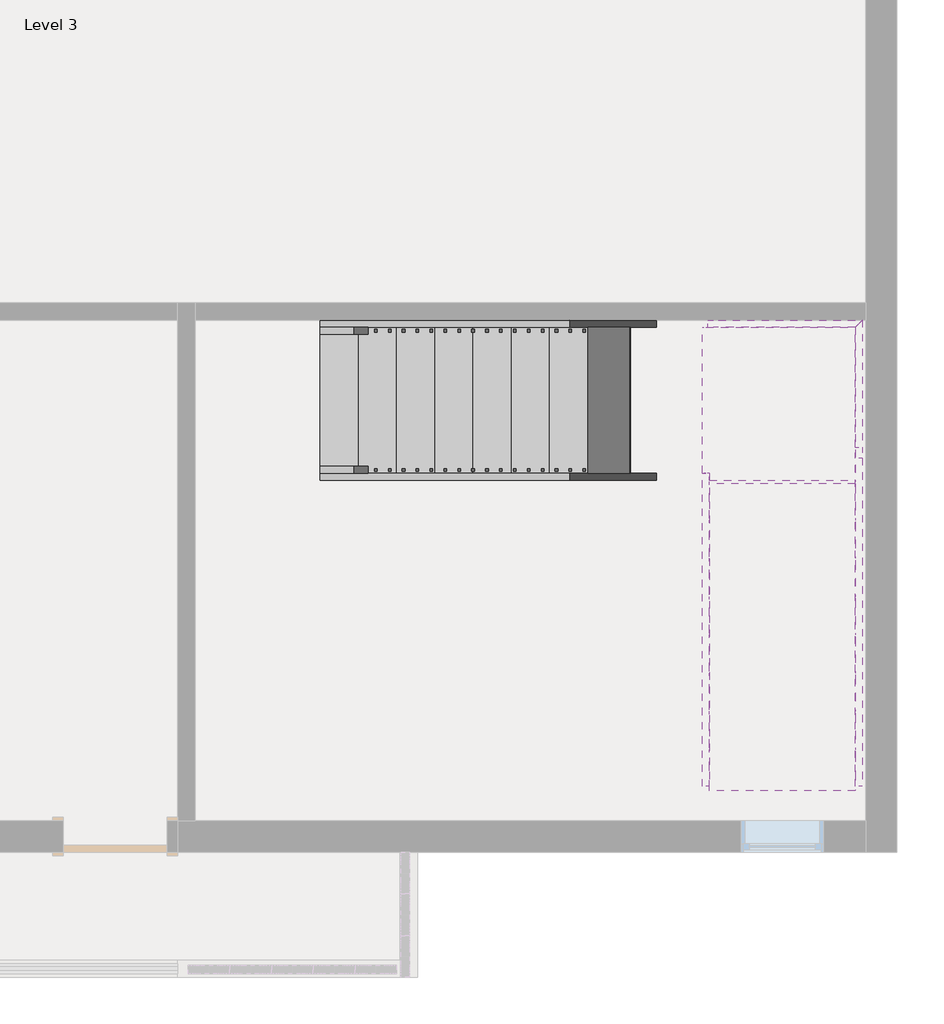
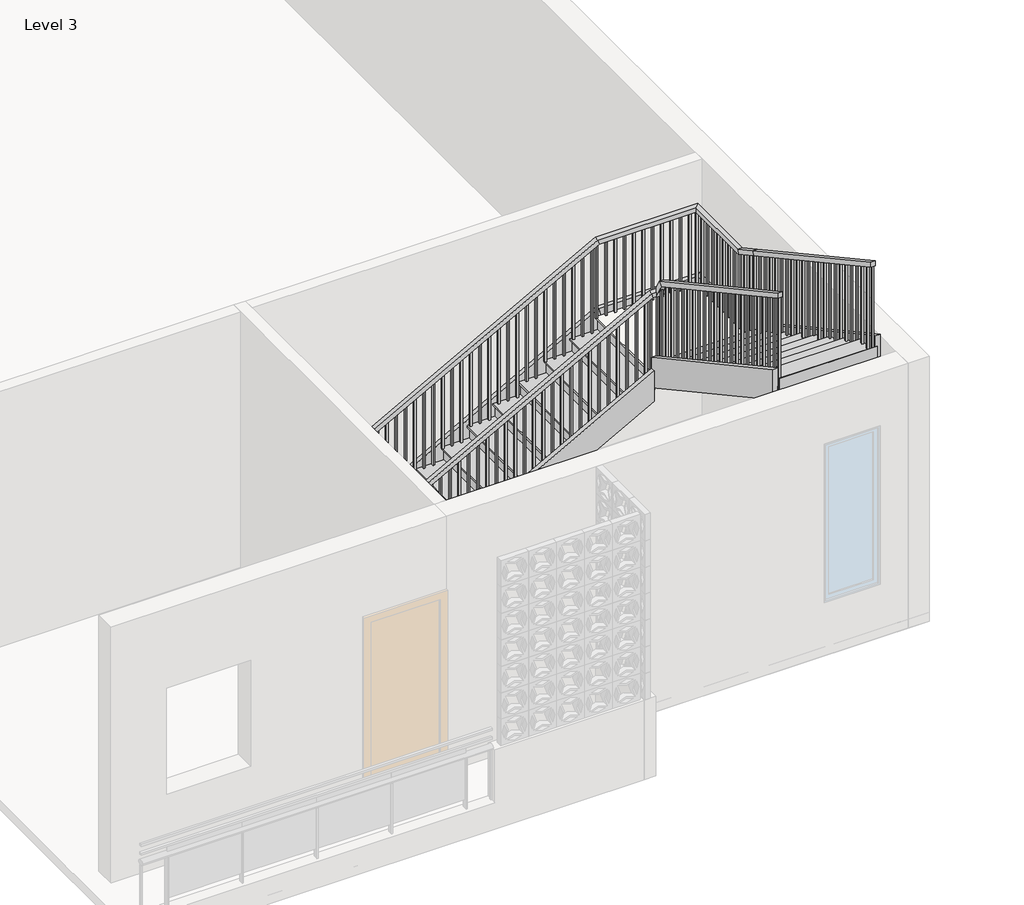
# One storey, part 2 of 2: 6 members, 2 railings, 2 stair flights, 1 slab.
"""IFC4 building model written with IfcOpenShell, lengths in millimetres."""

from ifc_helpers import new_model, si_unit, frame, origin, place, context, project, spatial, polyline, outline, extrude, faceted_brep, transform, mapped, element, save
from components import non_monolithic_landing_ee32a08e, stair_flight_b15b2b3c, stair_flight_a6ac55d9

model = new_model("IFC4")

# Units and contexts
model_context = context("Model", 3, world=origin())
ifc_project = project(units=[si_unit("LENGTHUNIT", "METRE", prefix="MILLI")], contexts=[model_context])

# Site, building, storey
site = spatial("IfcSite", under=ifc_project)
building = spatial("IfcBuilding", under=site)
storey = spatial("IfcBuildingStorey", under=building, Name="Level 3", Elevation=6096.0)

# Members
placement = place(None, origin())
element("IfcMember", 1, ObjectType="Stringer - 2\" Width", at=placement, inside=storey, context=model_context, shape_type="SweptSolid", body=[
    extrude(outline(polyline([(6302.7436667, -459.26646), (6096.0, -459.26646), (6096.0, -201.7743401), (7543.8, 2452.5256599), (7848.6, 2374.8034844), (6302.7436667, -459.26646)])), frame((0.0, -782.3834702, 0.0), z_axis=(0.0, 1.0, 0.0), x_axis=(0.0, 0.0, 1.0)), (0.0, 0.0, 1.0), 50.8),
])
element("IfcMember", 2, ObjectType="Stringer - 2\" Width", at=placement, inside=storey, context=model_context, shape_type="SweptSolid", body=[
    extrude(outline(polyline([(6302.7436667, -459.26646), (6096.0, -459.26646), (6096.0, -201.7743401), (7479.5497528, 2334.73354), (7826.7436667, 2334.73354), (6302.7436667, -459.26646)])), frame((0.0, -1899.9834702, 0.0), z_axis=(0.0, 1.0, 0.0), x_axis=(0.0, 0.0, 1.0)), (0.0, 0.0, 1.0), 50.8),
])
element("IfcMember", 3, ObjectType="Stringer - 2\" Width", at=placement, inside=storey, context=model_context, shape_type="SweptSolid", body=[
    extrude(outline(polyline([(-1660.6534146, 7848.6), (-1738.3755901, 7543.8), (-4135.1834702, 8851.1497528), (-4135.1834702, 9198.3436667), (-1660.6534146, 7848.6)])), frame((3452.33354, 0.0, 0.0), z_axis=(1.0, 0.0, 0.0), x_axis=(0.0, 1.0, 0.0)), (0.0, 0.0, 1.0), 50.8),
])
element("IfcMember", 4, ObjectType="Stringer - 2\" Width", at=placement, inside=storey, context=model_context, shape_type="SweptSolid", body=[
    extrude(outline(polyline([(-1849.1834702, 7951.4345758), (-1849.1834702, 7604.2406619), (-4135.1834702, 8851.1497528), (-4135.1834702, 9198.3436667), (-1849.1834702, 7951.4345758)])), frame((2334.73354, 0.0, 0.0), z_axis=(1.0, 0.0, 0.0), x_axis=(0.0, 1.0, 0.0)), (0.0, 0.0, 1.0), 50.8),
])
element("IfcMember", 5, ObjectType="Stringer - 2\" Width", at=placement, inside=storey, context=model_context, shape_type="Brep", body=[
    faceted_brep([(3452.33354, -1660.6534146, 7848.6), (3503.13354, -1660.6534146, 7848.6), (3503.13354, -731.5834702, 7848.6), (3452.33354, -782.3834702, 7848.6), (3452.33354, -1738.3755901, 7543.8), (3452.33354, -782.3834702, 7543.8), (3503.13354, -1738.3755901, 7543.8), (3503.13354, -731.5834702, 7543.8)], [[[0, 1, 2, 3]], [[4, 0, 3, 5]], [[6, 4, 5, 7]], [[1, 6, 7, 2]], [[1, 0, 4, 6]], [[2, 7, 5, 3]]]),
])
element("IfcMember", 6, ObjectType="Stringer - 2\" Width", at=placement, inside=storey, context=model_context, shape_type="Brep", body=[
    faceted_brep([(3452.33354, -782.3834702, 7848.6), (3503.13354, -731.5834702, 7848.6), (2374.8034844, -731.5834702, 7848.6), (2374.8034844, -782.3834702, 7848.6), (3452.33354, -782.3834702, 7543.8), (2452.5256599, -782.3834702, 7543.8), (3503.13354, -731.5834702, 7543.8), (2452.5256599, -731.5834702, 7543.8)], [[[0, 1, 2, 3]], [[4, 0, 3, 5]], [[6, 4, 5, 7]], [[1, 6, 7, 2]], [[1, 0, 4, 6]], [[2, 7, 5, 3]]]),
])

# Railings
element("IfcRailing", 7, ObjectType="Handrail - Rectangular", at=placement, inside=storey, context=model_context, shape_type="SolidModel", body=[
    faceted_brep([(-459.26646, -1798.3834702, 7162.8), (-459.26646, -1798.3834702, 7104.9343477), (-459.26646, -1849.1834702, 7104.9343477), (-459.26646, -1849.1834702, 7162.8), (2334.73354, -1798.3834702, 8686.8), (2347.687236, -1798.3834702, 8636.0), (2347.687236, -1849.1834702, 8636.0), (2334.73354, -1849.1834702, 8686.8), (2436.33354, -1798.3834702, 8686.8), (2436.33354, -1849.1834702, 8686.8), (2436.33354, -1849.1834702, 8636.0), (2436.33354, -1798.3834702, 8636.0)], [[[0, 1, 2, 3]], [[1, 0, 4, 5]], [[2, 1, 5, 6]], [[3, 2, 6, 7]], [[0, 3, 7, 4]], [[8, 9, 10, 11]], [[5, 4, 8, 11]], [[6, 5, 11, 10]], [[7, 6, 10, 9]], [[4, 7, 9, 8]]]),
    faceted_brep([(2436.33354, -1849.1834702, 8737.6), (2436.33354, -1849.1834702, 8624.0077467), (2385.53354, -1849.1834702, 8624.0077467), (2385.53354, -1849.1834702, 8737.6), (2436.33354, -1899.9834702, 8839.2), (2436.33354, -1938.2955084, 8802.231823), (2385.53354, -1938.2955084, 8802.231823), (2385.53354, -1899.9834702, 8839.2), (2436.33354, -4135.1834702, 10058.4), (2385.53354, -4135.1834702, 10058.4), (2385.53354, -4135.1834702, 10000.5343477), (2436.33354, -4135.1834702, 10000.5343477)], [[[0, 1, 2, 3]], [[1, 0, 4, 5]], [[2, 1, 5, 6]], [[3, 2, 6, 7]], [[0, 3, 7, 4]], [[8, 9, 10, 11]], [[5, 4, 8, 11]], [[6, 5, 11, 10]], [[7, 6, 10, 9]], [[4, 7, 9, 8]]]),
    extrude(outline(polyline([(-4043.1084702, 9950.3116204), (-4024.0584702, 9939.9207113), (-4024.0584702, 8991.6), (-4043.1084702, 8991.6), (-4043.1084702, 9950.3116204)])), frame((2401.40854, 0.0, 0.0), z_axis=(1.0, 0.0, 0.0), x_axis=(0.0, 1.0, 0.0)), (0.0, 0.0, 1.0), 19.05),
    extrude(outline(polyline([(-3941.5084702, 9894.8934386), (-3922.4584702, 9884.5025295), (-3922.4584702, 8991.6), (-3941.5084702, 8991.6), (-3941.5084702, 9894.8934386)])), frame((2401.40854, 0.0, 0.0), z_axis=(1.0, 0.0, 0.0), x_axis=(0.0, 1.0, 0.0)), (0.0, 0.0, 1.0), 19.05),
    extrude(outline(polyline([(-3839.9084702, 9839.4752568), (-3820.8584702, 9829.0843477), (-3820.8584702, 8839.2), (-3839.9084702, 8839.2), (-3839.9084702, 9839.4752568)])), frame((2401.40854, 0.0, 0.0), z_axis=(1.0, 0.0, 0.0), x_axis=(0.0, 1.0, 0.0)), (0.0, 0.0, 1.0), 19.05),
    extrude(outline(polyline([(-3738.3084702, 9784.0570749), (-3719.2584702, 9773.6661659), (-3719.2584702, 8839.2), (-3738.3084702, 8839.2), (-3738.3084702, 9784.0570749)])), frame((2401.40854, 0.0, 0.0), z_axis=(1.0, 0.0, 0.0), x_axis=(0.0, 1.0, 0.0)), (0.0, 0.0, 1.0), 19.05),
    extrude(outline(polyline([(-3636.7084702, 9728.6388931), (-3617.6584702, 9718.247984), (-3617.6584702, 8839.2), (-3636.7084702, 8839.2), (-3636.7084702, 9728.6388931)])), frame((2401.40854, 0.0, 0.0), z_axis=(1.0, 0.0, 0.0), x_axis=(0.0, 1.0, 0.0)), (0.0, 0.0, 1.0), 19.05),
    extrude(outline(polyline([(-3535.1084702, 9673.2207113), (-3516.0584702, 9662.8298022), (-3516.0584702, 8686.8), (-3535.1084702, 8686.8), (-3535.1084702, 9673.2207113)])), frame((2401.40854, 0.0, 0.0), z_axis=(1.0, 0.0, 0.0), x_axis=(0.0, 1.0, 0.0)), (0.0, 0.0, 1.0), 19.05),
    extrude(outline(polyline([(-3433.5084702, 9617.8025295), (-3414.4584702, 9607.4116204), (-3414.4584702, 8686.8), (-3433.5084702, 8686.8), (-3433.5084702, 9617.8025295)])), frame((2401.40854, 0.0, 0.0), z_axis=(1.0, 0.0, 0.0), x_axis=(0.0, 1.0, 0.0)), (0.0, 0.0, 1.0), 19.05),
    extrude(outline(polyline([(-3331.9084702, 9562.3843477), (-3312.8584702, 9551.9934386), (-3312.8584702, 8686.8), (-3331.9084702, 8686.8), (-3331.9084702, 9562.3843477)])), frame((2401.40854, 0.0, 0.0), z_axis=(1.0, 0.0, 0.0), x_axis=(0.0, 1.0, 0.0)), (0.0, 0.0, 1.0), 19.05),
    extrude(outline(polyline([(-3230.3084702, 9506.9661659), (-3211.2584702, 9496.5752568), (-3211.2584702, 8534.4), (-3230.3084702, 8534.4), (-3230.3084702, 9506.9661659)])), frame((2401.40854, 0.0, 0.0), z_axis=(1.0, 0.0, 0.0), x_axis=(0.0, 1.0, 0.0)), (0.0, 0.0, 1.0), 19.05),
    extrude(outline(polyline([(-3128.7084702, 9451.547984), (-3109.6584702, 9441.1570749), (-3109.6584702, 8534.4), (-3128.7084702, 8534.4), (-3128.7084702, 9451.547984)])), frame((2401.40854, 0.0, 0.0), z_axis=(1.0, 0.0, 0.0), x_axis=(0.0, 1.0, 0.0)), (0.0, 0.0, 1.0), 19.05),
    extrude(outline(polyline([(-3027.1084702, 9396.1298022), (-3008.0584702, 9385.7388931), (-3008.0584702, 8534.4), (-3027.1084702, 8534.4), (-3027.1084702, 9396.1298022)])), frame((2401.40854, 0.0, 0.0), z_axis=(1.0, 0.0, 0.0), x_axis=(0.0, 1.0, 0.0)), (0.0, 0.0, 1.0), 19.05),
    extrude(outline(polyline([(-2925.5084702, 9340.7116204), (-2906.4584702, 9330.3207113), (-2906.4584702, 8382.0), (-2925.5084702, 8382.0), (-2925.5084702, 9340.7116204)])), frame((2401.40854, 0.0, 0.0), z_axis=(1.0, 0.0, 0.0), x_axis=(0.0, 1.0, 0.0)), (0.0, 0.0, 1.0), 19.05),
    extrude(outline(polyline([(-2823.9084702, 9285.2934386), (-2804.8584702, 9274.9025295), (-2804.8584702, 8382.0), (-2823.9084702, 8382.0), (-2823.9084702, 9285.2934386)])), frame((2401.40854, 0.0, 0.0), z_axis=(1.0, 0.0, 0.0), x_axis=(0.0, 1.0, 0.0)), (0.0, 0.0, 1.0), 19.05),
    extrude(outline(polyline([(-2722.3084702, 9229.8752568), (-2703.2584702, 9219.4843477), (-2703.2584702, 8229.6), (-2722.3084702, 8229.6), (-2722.3084702, 9229.8752568)])), frame((2401.40854, 0.0, 0.0), z_axis=(1.0, 0.0, 0.0), x_axis=(0.0, 1.0, 0.0)), (0.0, 0.0, 1.0), 19.05),
    extrude(outline(polyline([(-2620.7084702, 9174.4570749), (-2601.6584702, 9164.0661659), (-2601.6584702, 8229.6), (-2620.7084702, 8229.6), (-2620.7084702, 9174.4570749)])), frame((2401.40854, 0.0, 0.0), z_axis=(1.0, 0.0, 0.0), x_axis=(0.0, 1.0, 0.0)), (0.0, 0.0, 1.0), 19.05),
    extrude(outline(polyline([(-2519.1084702, 9119.0388931), (-2500.0584702, 9108.647984), (-2500.0584702, 8229.6), (-2519.1084702, 8229.6), (-2519.1084702, 9119.0388931)])), frame((2401.40854, 0.0, 0.0), z_axis=(1.0, 0.0, 0.0), x_axis=(0.0, 1.0, 0.0)), (0.0, 0.0, 1.0), 19.05),
    extrude(outline(polyline([(-2417.5084702, 9063.6207113), (-2398.4584702, 9053.2298022), (-2398.4584702, 8077.2), (-2417.5084702, 8077.2), (-2417.5084702, 9063.6207113)])), frame((2401.40854, 0.0, 0.0), z_axis=(1.0, 0.0, 0.0), x_axis=(0.0, 1.0, 0.0)), (0.0, 0.0, 1.0), 19.05),
    extrude(outline(polyline([(-2315.9084702, 9008.2025295), (-2296.8584702, 8997.8116204), (-2296.8584702, 8077.2), (-2315.9084702, 8077.2), (-2315.9084702, 9008.2025295)])), frame((2401.40854, 0.0, 0.0), z_axis=(1.0, 0.0, 0.0), x_axis=(0.0, 1.0, 0.0)), (0.0, 0.0, 1.0), 19.05),
    extrude(outline(polyline([(-2214.3084702, 8952.7843477), (-2195.2584702, 8942.3934386), (-2195.2584702, 8077.2), (-2214.3084702, 8077.2), (-2214.3084702, 8952.7843477)])), frame((2401.40854, 0.0, 0.0), z_axis=(1.0, 0.0, 0.0), x_axis=(0.0, 1.0, 0.0)), (0.0, 0.0, 1.0), 19.05),
    extrude(outline(polyline([(-2112.7084702, 8897.3661659), (-2093.6584702, 8886.9752568), (-2093.6584702, 7924.8), (-2112.7084702, 7924.8), (-2112.7084702, 8897.3661659)])), frame((2401.40854, 0.0, 0.0), z_axis=(1.0, 0.0, 0.0), x_axis=(0.0, 1.0, 0.0)), (0.0, 0.0, 1.0), 19.05),
    extrude(outline(polyline([(-2011.1084702, 8841.947984), (-1992.0584702, 8831.5570749), (-1992.0584702, 7924.8), (-2011.1084702, 7924.8), (-2011.1084702, 8841.947984)])), frame((2401.40854, 0.0, 0.0), z_axis=(1.0, 0.0, 0.0), x_axis=(0.0, 1.0, 0.0)), (0.0, 0.0, 1.0), 19.05),
    extrude(outline(polyline([(8606.4207113, 2293.45854), (8596.0298022, 2274.40854), (7620.0, 2274.40854), (7620.0, 2293.45854), (8606.4207113, 2293.45854)])), frame((0.0, -1833.3084702, 0.0), z_axis=(0.0, 1.0, 0.0), x_axis=(0.0, 0.0, 1.0)), (0.0, 0.0, 1.0), 19.05),
    extrude(outline(polyline([(8551.0025295, 2191.85854), (8540.6116204, 2172.80854), (7620.0, 2172.80854), (7620.0, 2191.85854), (8551.0025295, 2191.85854)])), frame((0.0, -1833.3084702, 0.0), z_axis=(0.0, 1.0, 0.0), x_axis=(0.0, 0.0, 1.0)), (0.0, 0.0, 1.0), 19.05),
    extrude(outline(polyline([(8495.5843477, 2090.25854), (8485.1934386, 2071.20854), (7620.0, 2071.20854), (7620.0, 2090.25854), (8495.5843477, 2090.25854)])), frame((0.0, -1833.3084702, 0.0), z_axis=(0.0, 1.0, 0.0), x_axis=(0.0, 0.0, 1.0)), (0.0, 0.0, 1.0), 19.05),
    extrude(outline(polyline([(8440.1661659, 1988.65854), (8429.7752568, 1969.60854), (7467.6, 1969.60854), (7467.6, 1988.65854), (8440.1661659, 1988.65854)])), frame((0.0, -1833.3084702, 0.0), z_axis=(0.0, 1.0, 0.0), x_axis=(0.0, 0.0, 1.0)), (0.0, 0.0, 1.0), 19.05),
    extrude(outline(polyline([(8384.747984, 1887.05854), (8374.3570749, 1868.00854), (7467.6, 1868.00854), (7467.6, 1887.05854), (8384.747984, 1887.05854)])), frame((0.0, -1833.3084702, 0.0), z_axis=(0.0, 1.0, 0.0), x_axis=(0.0, 0.0, 1.0)), (0.0, 0.0, 1.0), 19.05),
    extrude(outline(polyline([(8329.3298022, 1785.45854), (8318.9388931, 1766.40854), (7467.6, 1766.40854), (7467.6, 1785.45854), (8329.3298022, 1785.45854)])), frame((0.0, -1833.3084702, 0.0), z_axis=(0.0, 1.0, 0.0), x_axis=(0.0, 0.0, 1.0)), (0.0, 0.0, 1.0), 19.05),
    extrude(outline(polyline([(8273.9116204, 1683.85854), (8263.5207113, 1664.80854), (7315.2, 1664.80854), (7315.2, 1683.85854), (8273.9116204, 1683.85854)])), frame((0.0, -1833.3084702, 0.0), z_axis=(0.0, 1.0, 0.0), x_axis=(0.0, 0.0, 1.0)), (0.0, 0.0, 1.0), 19.05),
    extrude(outline(polyline([(8218.4934386, 1582.25854), (8208.1025295, 1563.20854), (7315.2, 1563.20854), (7315.2, 1582.25854), (8218.4934386, 1582.25854)])), frame((0.0, -1833.3084702, 0.0), z_axis=(0.0, 1.0, 0.0), x_axis=(0.0, 0.0, 1.0)), (0.0, 0.0, 1.0), 19.05),
    extrude(outline(polyline([(8163.0752568, 1480.65854), (8152.6843477, 1461.60854), (7162.8, 1461.60854), (7162.8, 1480.65854), (8163.0752568, 1480.65854)])), frame((0.0, -1833.3084702, 0.0), z_axis=(0.0, 1.0, 0.0), x_axis=(0.0, 0.0, 1.0)), (0.0, 0.0, 1.0), 19.05),
    extrude(outline(polyline([(8107.6570749, 1379.05854), (8097.2661659, 1360.00854), (7162.8, 1360.00854), (7162.8, 1379.05854), (8107.6570749, 1379.05854)])), frame((0.0, -1833.3084702, 0.0), z_axis=(0.0, 1.0, 0.0), x_axis=(0.0, 0.0, 1.0)), (0.0, 0.0, 1.0), 19.05),
    extrude(outline(polyline([(8052.2388931, 1277.45854), (8041.847984, 1258.40854), (7162.8, 1258.40854), (7162.8, 1277.45854), (8052.2388931, 1277.45854)])), frame((0.0, -1833.3084702, 0.0), z_axis=(0.0, 1.0, 0.0), x_axis=(0.0, 0.0, 1.0)), (0.0, 0.0, 1.0), 19.05),
    extrude(outline(polyline([(7996.8207113, 1175.85854), (7986.4298022, 1156.80854), (7010.4, 1156.80854), (7010.4, 1175.85854), (7996.8207113, 1175.85854)])), frame((0.0, -1833.3084702, 0.0), z_axis=(0.0, 1.0, 0.0), x_axis=(0.0, 0.0, 1.0)), (0.0, 0.0, 1.0), 19.05),
    extrude(outline(polyline([(7941.4025295, 1074.25854), (7931.0116204, 1055.20854), (7010.4, 1055.20854), (7010.4, 1074.25854), (7941.4025295, 1074.25854)])), frame((0.0, -1833.3084702, 0.0), z_axis=(0.0, 1.0, 0.0), x_axis=(0.0, 0.0, 1.0)), (0.0, 0.0, 1.0), 19.05),
    extrude(outline(polyline([(7885.9843477, 972.65854), (7875.5934386, 953.60854), (7010.4, 953.60854), (7010.4, 972.65854), (7885.9843477, 972.65854)])), frame((0.0, -1833.3084702, 0.0), z_axis=(0.0, 1.0, 0.0), x_axis=(0.0, 0.0, 1.0)), (0.0, 0.0, 1.0), 19.05),
    extrude(outline(polyline([(7830.5661659, 871.05854), (7820.1752568, 852.00854), (6858.0, 852.00854), (6858.0, 871.05854), (7830.5661659, 871.05854)])), frame((0.0, -1833.3084702, 0.0), z_axis=(0.0, 1.0, 0.0), x_axis=(0.0, 0.0, 1.0)), (0.0, 0.0, 1.0), 19.05),
    extrude(outline(polyline([(7775.147984, 769.45854), (7764.7570749, 750.40854), (6858.0, 750.40854), (6858.0, 769.45854), (7775.147984, 769.45854)])), frame((0.0, -1833.3084702, 0.0), z_axis=(0.0, 1.0, 0.0), x_axis=(0.0, 0.0, 1.0)), (0.0, 0.0, 1.0), 19.05),
    extrude(outline(polyline([(7719.7298022, 667.85854), (7709.3388931, 648.80854), (6858.0, 648.80854), (6858.0, 667.85854), (7719.7298022, 667.85854)])), frame((0.0, -1833.3084702, 0.0), z_axis=(0.0, 1.0, 0.0), x_axis=(0.0, 0.0, 1.0)), (0.0, 0.0, 1.0), 19.05),
    extrude(outline(polyline([(7664.3116204, 566.25854), (7653.9207113, 547.20854), (6705.6, 547.20854), (6705.6, 566.25854), (7664.3116204, 566.25854)])), frame((0.0, -1833.3084702, 0.0), z_axis=(0.0, 1.0, 0.0), x_axis=(0.0, 0.0, 1.0)), (0.0, 0.0, 1.0), 19.05),
    extrude(outline(polyline([(7608.8934386, 464.65854), (7598.5025295, 445.60854), (6705.6, 445.60854), (6705.6, 464.65854), (7608.8934386, 464.65854)])), frame((0.0, -1833.3084702, 0.0), z_axis=(0.0, 1.0, 0.0), x_axis=(0.0, 0.0, 1.0)), (0.0, 0.0, 1.0), 19.05),
    extrude(outline(polyline([(7553.4752568, 363.05854), (7543.0843477, 344.00854), (6553.2, 344.00854), (6553.2, 363.05854), (7553.4752568, 363.05854)])), frame((0.0, -1833.3084702, 0.0), z_axis=(0.0, 1.0, 0.0), x_axis=(0.0, 0.0, 1.0)), (0.0, 0.0, 1.0), 19.05),
    extrude(outline(polyline([(7498.0570749, 261.45854), (7487.6661659, 242.40854), (6553.2, 242.40854), (6553.2, 261.45854), (7498.0570749, 261.45854)])), frame((0.0, -1833.3084702, 0.0), z_axis=(0.0, 1.0, 0.0), x_axis=(0.0, 0.0, 1.0)), (0.0, 0.0, 1.0), 19.05),
    extrude(outline(polyline([(7442.6388931, 159.85854), (7432.247984, 140.80854), (6553.2, 140.80854), (6553.2, 159.85854), (7442.6388931, 159.85854)])), frame((0.0, -1833.3084702, 0.0), z_axis=(0.0, 1.0, 0.0), x_axis=(0.0, 0.0, 1.0)), (0.0, 0.0, 1.0), 19.05),
    extrude(outline(polyline([(7387.2207113, 58.25854), (7376.8298022, 39.20854), (6400.8, 39.20854), (6400.8, 58.25854), (7387.2207113, 58.25854)])), frame((0.0, -1833.3084702, 0.0), z_axis=(0.0, 1.0, 0.0), x_axis=(0.0, 0.0, 1.0)), (0.0, 0.0, 1.0), 19.05),
    extrude(outline(polyline([(7331.8025295, -43.34146), (7321.4116204, -62.39146), (6400.8, -62.39146), (6400.8, -43.34146), (7331.8025295, -43.34146)])), frame((0.0, -1833.3084702, 0.0), z_axis=(0.0, 1.0, 0.0), x_axis=(0.0, 0.0, 1.0)), (0.0, 0.0, 1.0), 19.05),
    extrude(outline(polyline([(7276.3843477, -144.94146), (7265.9934386, -163.99146), (6400.8, -163.99146), (6400.8, -144.94146), (7276.3843477, -144.94146)])), frame((0.0, -1833.3084702, 0.0), z_axis=(0.0, 1.0, 0.0), x_axis=(0.0, 0.0, 1.0)), (0.0, 0.0, 1.0), 19.05),
    extrude(outline(polyline([(7220.9661659, -246.54146), (7210.5752568, -265.59146), (6248.4, -265.59146), (6248.4, -246.54146), (7220.9661659, -246.54146)])), frame((0.0, -1833.3084702, 0.0), z_axis=(0.0, 1.0, 0.0), x_axis=(0.0, 0.0, 1.0)), (0.0, 0.0, 1.0), 19.05),
    extrude(outline(polyline([(7165.547984, -348.14146), (7155.1570749, -367.19146), (6248.4, -367.19146), (6248.4, -348.14146), (7165.547984, -348.14146)])), frame((0.0, -1833.3084702, 0.0), z_axis=(0.0, 1.0, 0.0), x_axis=(0.0, 0.0, 1.0)), (0.0, 0.0, 1.0), 19.05),
    extrude(outline(polyline([(-1909.5084702, 8744.6577467), (-1890.4584702, 8706.5577467), (-1890.4584702, 7772.4), (-1909.5084702, 7772.4), (-1909.5084702, 8744.6577467)])), frame((2401.40854, 0.0, 0.0), z_axis=(1.0, 0.0, 0.0), x_axis=(0.0, 1.0, 0.0)), (0.0, 0.0, 1.0), 19.05),
    extrude(outline(polyline([(2401.40854, -1833.3084702), (2401.40854, -1814.2584702), (2420.45854, -1814.2584702), (2420.45854, -1833.3084702), (2401.40854, -1833.3084702)])), frame((0.0, 0.0, 7772.4), z_axis=(0.0, 0.0, 1.0), x_axis=(1.0, 0.0, 0.0)), (0.0, 0.0, 1.0), 863.6),
    extrude(outline(polyline([(8634.1298022, 2344.25854), (8623.7388931, 2325.20854), (7772.4, 2325.20854), (7772.4, 2344.25854), (8634.1298022, 2344.25854)])), frame((0.0, -1833.3084702, 0.0), z_axis=(0.0, 1.0, 0.0), x_axis=(0.0, 0.0, 1.0)), (0.0, 0.0, 1.0), 19.05),
    extrude(outline(polyline([(-4135.1834702, 10000.5343477), (-4116.1334702, 9990.1434386), (-4116.1334702, 8991.6), (-4135.1834702, 8991.6), (-4135.1834702, 10000.5343477)])), frame((2401.40854, 0.0, 0.0), z_axis=(1.0, 0.0, 0.0), x_axis=(0.0, 1.0, 0.0)), (0.0, 0.0, 1.0), 19.05),
    extrude(outline(polyline([(7115.3252568, -440.21646), (7104.9343477, -459.26646), (6248.4, -459.26646), (6248.4, -440.21646), (7115.3252568, -440.21646)])), frame((0.0, -1833.3084702, 0.0), z_axis=(0.0, 1.0, 0.0), x_axis=(0.0, 0.0, 1.0)), (0.0, 0.0, 1.0), 19.05),
])
element("IfcRailing", 8, ObjectType="Handrail - Rectangular", at=placement, inside=storey, context=model_context, shape_type="SolidModel", body=[
    faceted_brep([(-459.26646, -782.3834702, 7162.8), (-459.26646, -782.3834702, 7104.9343477), (-459.26646, -833.1834702, 7104.9343477), (-459.26646, -833.1834702, 7162.8), (2334.73354, -782.3834702, 8686.8), (2347.687236, -782.3834702, 8636.0), (2347.687236, -833.1834702, 8636.0), (2334.73354, -833.1834702, 8686.8), (3452.33354, -782.3834702, 8686.8), (3452.33354, -782.3834702, 8636.0), (3401.53354, -833.1834702, 8636.0), (3401.53354, -833.1834702, 8686.8), (3452.33354, -1620.5834702, 8686.8), (3452.33354, -1633.5371661, 8636.0), (3401.53354, -1633.5371661, 8636.0), (3401.53354, -1620.5834702, 8686.8), (3452.33354, -1899.9834702, 8839.2), (3452.33354, -1924.3091585, 8794.6029049), (3401.53354, -1924.3091585, 8794.6029049), (3401.53354, -1899.9834702, 8839.2), (3452.33354, -4135.1834702, 10058.4), (3401.53354, -4135.1834702, 10058.4), (3401.53354, -4135.1834702, 10000.5343477), (3452.33354, -4135.1834702, 10000.5343477)], [[[0, 1, 2, 3]], [[1, 0, 4, 5]], [[2, 1, 5, 6]], [[3, 2, 6, 7]], [[0, 3, 7, 4]], [[5, 4, 8, 9]], [[6, 5, 9, 10]], [[7, 6, 10, 11]], [[4, 7, 11, 8]], [[9, 8, 12, 13]], [[10, 9, 13, 14]], [[11, 10, 14, 15]], [[8, 11, 15, 12]], [[13, 12, 16, 17]], [[14, 13, 17, 18]], [[15, 14, 18, 19]], [[12, 15, 19, 16]], [[20, 21, 22, 23]], [[17, 16, 20, 23]], [[18, 17, 23, 22]], [[19, 18, 22, 21]], [[16, 19, 21, 20]]]),
    extrude(outline(polyline([(-4024.0584702, 9939.9207113), (-4024.0584702, 8991.6), (-4043.1084702, 8991.6), (-4043.1084702, 9950.3116204), (-4024.0584702, 9939.9207113)])), frame((3417.40854, 0.0, 0.0), z_axis=(1.0, 0.0, 0.0), x_axis=(0.0, 1.0, 0.0)), (0.0, 0.0, 1.0), 19.05),
    extrude(outline(polyline([(-3922.4584702, 9884.5025295), (-3922.4584702, 8991.6), (-3941.5084702, 8991.6), (-3941.5084702, 9894.8934386), (-3922.4584702, 9884.5025295)])), frame((3417.40854, 0.0, 0.0), z_axis=(1.0, 0.0, 0.0), x_axis=(0.0, 1.0, 0.0)), (0.0, 0.0, 1.0), 19.05),
    extrude(outline(polyline([(-3820.8584702, 9829.0843477), (-3820.8584702, 8839.2), (-3839.9084702, 8839.2), (-3839.9084702, 9839.4752568), (-3820.8584702, 9829.0843477)])), frame((3417.40854, 0.0, 0.0), z_axis=(1.0, 0.0, 0.0), x_axis=(0.0, 1.0, 0.0)), (0.0, 0.0, 1.0), 19.05),
    extrude(outline(polyline([(-3719.2584702, 9773.6661659), (-3719.2584702, 8839.2), (-3738.3084702, 8839.2), (-3738.3084702, 9784.0570749), (-3719.2584702, 9773.6661659)])), frame((3417.40854, 0.0, 0.0), z_axis=(1.0, 0.0, 0.0), x_axis=(0.0, 1.0, 0.0)), (0.0, 0.0, 1.0), 19.05),
    extrude(outline(polyline([(-3617.6584702, 9718.247984), (-3617.6584702, 8839.2), (-3636.7084702, 8839.2), (-3636.7084702, 9728.6388931), (-3617.6584702, 9718.247984)])), frame((3417.40854, 0.0, 0.0), z_axis=(1.0, 0.0, 0.0), x_axis=(0.0, 1.0, 0.0)), (0.0, 0.0, 1.0), 19.05),
    extrude(outline(polyline([(-3516.0584702, 9662.8298022), (-3516.0584702, 8686.8), (-3535.1084702, 8686.8), (-3535.1084702, 9673.2207113), (-3516.0584702, 9662.8298022)])), frame((3417.40854, 0.0, 0.0), z_axis=(1.0, 0.0, 0.0), x_axis=(0.0, 1.0, 0.0)), (0.0, 0.0, 1.0), 19.05),
    extrude(outline(polyline([(-3414.4584702, 9607.4116204), (-3414.4584702, 8686.8), (-3433.5084702, 8686.8), (-3433.5084702, 9617.8025295), (-3414.4584702, 9607.4116204)])), frame((3417.40854, 0.0, 0.0), z_axis=(1.0, 0.0, 0.0), x_axis=(0.0, 1.0, 0.0)), (0.0, 0.0, 1.0), 19.05),
    extrude(outline(polyline([(-3312.8584702, 9551.9934386), (-3312.8584702, 8686.8), (-3331.9084702, 8686.8), (-3331.9084702, 9562.3843477), (-3312.8584702, 9551.9934386)])), frame((3417.40854, 0.0, 0.0), z_axis=(1.0, 0.0, 0.0), x_axis=(0.0, 1.0, 0.0)), (0.0, 0.0, 1.0), 19.05),
    extrude(outline(polyline([(-3211.2584702, 9496.5752568), (-3211.2584702, 8534.4), (-3230.3084702, 8534.4), (-3230.3084702, 9506.9661659), (-3211.2584702, 9496.5752568)])), frame((3417.40854, 0.0, 0.0), z_axis=(1.0, 0.0, 0.0), x_axis=(0.0, 1.0, 0.0)), (0.0, 0.0, 1.0), 19.05),
    extrude(outline(polyline([(-3109.6584702, 9441.1570749), (-3109.6584702, 8534.4), (-3128.7084702, 8534.4), (-3128.7084702, 9451.547984), (-3109.6584702, 9441.1570749)])), frame((3417.40854, 0.0, 0.0), z_axis=(1.0, 0.0, 0.0), x_axis=(0.0, 1.0, 0.0)), (0.0, 0.0, 1.0), 19.05),
    extrude(outline(polyline([(-3008.0584702, 9385.7388931), (-3008.0584702, 8534.4), (-3027.1084702, 8534.4), (-3027.1084702, 9396.1298022), (-3008.0584702, 9385.7388931)])), frame((3417.40854, 0.0, 0.0), z_axis=(1.0, 0.0, 0.0), x_axis=(0.0, 1.0, 0.0)), (0.0, 0.0, 1.0), 19.05),
    extrude(outline(polyline([(-2906.4584702, 9330.3207113), (-2906.4584702, 8382.0), (-2925.5084702, 8382.0), (-2925.5084702, 9340.7116204), (-2906.4584702, 9330.3207113)])), frame((3417.40854, 0.0, 0.0), z_axis=(1.0, 0.0, 0.0), x_axis=(0.0, 1.0, 0.0)), (0.0, 0.0, 1.0), 19.05),
    extrude(outline(polyline([(-2804.8584702, 9274.9025295), (-2804.8584702, 8382.0), (-2823.9084702, 8382.0), (-2823.9084702, 9285.2934386), (-2804.8584702, 9274.9025295)])), frame((3417.40854, 0.0, 0.0), z_axis=(1.0, 0.0, 0.0), x_axis=(0.0, 1.0, 0.0)), (0.0, 0.0, 1.0), 19.05),
    extrude(outline(polyline([(-2703.2584702, 9219.4843477), (-2703.2584702, 8229.6), (-2722.3084702, 8229.6), (-2722.3084702, 9229.8752568), (-2703.2584702, 9219.4843477)])), frame((3417.40854, 0.0, 0.0), z_axis=(1.0, 0.0, 0.0), x_axis=(0.0, 1.0, 0.0)), (0.0, 0.0, 1.0), 19.05),
    extrude(outline(polyline([(-2601.6584702, 9164.0661659), (-2601.6584702, 8229.6), (-2620.7084702, 8229.6), (-2620.7084702, 9174.4570749), (-2601.6584702, 9164.0661659)])), frame((3417.40854, 0.0, 0.0), z_axis=(1.0, 0.0, 0.0), x_axis=(0.0, 1.0, 0.0)), (0.0, 0.0, 1.0), 19.05),
    extrude(outline(polyline([(-2500.0584702, 9108.647984), (-2500.0584702, 8229.6), (-2519.1084702, 8229.6), (-2519.1084702, 9119.0388931), (-2500.0584702, 9108.647984)])), frame((3417.40854, 0.0, 0.0), z_axis=(1.0, 0.0, 0.0), x_axis=(0.0, 1.0, 0.0)), (0.0, 0.0, 1.0), 19.05),
    extrude(outline(polyline([(-2398.4584702, 9053.2298022), (-2398.4584702, 8077.2), (-2417.5084702, 8077.2), (-2417.5084702, 9063.6207113), (-2398.4584702, 9053.2298022)])), frame((3417.40854, 0.0, 0.0), z_axis=(1.0, 0.0, 0.0), x_axis=(0.0, 1.0, 0.0)), (0.0, 0.0, 1.0), 19.05),
    extrude(outline(polyline([(-2296.8584702, 8997.8116204), (-2296.8584702, 8077.2), (-2315.9084702, 8077.2), (-2315.9084702, 9008.2025295), (-2296.8584702, 8997.8116204)])), frame((3417.40854, 0.0, 0.0), z_axis=(1.0, 0.0, 0.0), x_axis=(0.0, 1.0, 0.0)), (0.0, 0.0, 1.0), 19.05),
    extrude(outline(polyline([(-2195.2584702, 8942.3934386), (-2195.2584702, 8077.2), (-2214.3084702, 8077.2), (-2214.3084702, 8952.7843477), (-2195.2584702, 8942.3934386)])), frame((3417.40854, 0.0, 0.0), z_axis=(1.0, 0.0, 0.0), x_axis=(0.0, 1.0, 0.0)), (0.0, 0.0, 1.0), 19.05),
    extrude(outline(polyline([(-2093.6584702, 8886.9752568), (-2093.6584702, 7924.8), (-2112.7084702, 7924.8), (-2112.7084702, 8897.3661659), (-2093.6584702, 8886.9752568)])), frame((3417.40854, 0.0, 0.0), z_axis=(1.0, 0.0, 0.0), x_axis=(0.0, 1.0, 0.0)), (0.0, 0.0, 1.0), 19.05),
    extrude(outline(polyline([(-1992.0584702, 8831.5570749), (-1992.0584702, 7924.8), (-2011.1084702, 7924.8), (-2011.1084702, 8841.947984), (-1992.0584702, 8831.5570749)])), frame((3417.40854, 0.0, 0.0), z_axis=(1.0, 0.0, 0.0), x_axis=(0.0, 1.0, 0.0)), (0.0, 0.0, 1.0), 19.05),
    extrude(outline(polyline([(-1814.2584702, 8734.5752568), (-1814.2584702, 7772.4), (-1833.3084702, 7772.4), (-1833.3084702, 8744.9661659), (-1814.2584702, 8734.5752568)])), frame((3417.40854, 0.0, 0.0), z_axis=(1.0, 0.0, 0.0), x_axis=(0.0, 1.0, 0.0)), (0.0, 0.0, 1.0), 19.05),
    extrude(outline(polyline([(-1712.6584702, 8679.1570749), (-1712.6584702, 7772.4), (-1731.7084702, 7772.4), (-1731.7084702, 8689.547984), (-1712.6584702, 8679.1570749)])), frame((3417.40854, 0.0, 0.0), z_axis=(1.0, 0.0, 0.0), x_axis=(0.0, 1.0, 0.0)), (0.0, 0.0, 1.0), 19.05),
    extrude(outline(polyline([(3436.45854, -1611.0584702), (3436.45854, -1630.1084702), (3417.40854, -1630.1084702), (3417.40854, -1611.0584702), (3436.45854, -1611.0584702)])), frame((0.0, 0.0, 7772.4), z_axis=(0.0, 0.0, 1.0), x_axis=(1.0, 0.0, 0.0)), (0.0, 0.0, 1.0), 863.6),
    extrude(outline(polyline([(3436.45854, -1509.4584702), (3436.45854, -1528.5084702), (3417.40854, -1528.5084702), (3417.40854, -1509.4584702), (3436.45854, -1509.4584702)])), frame((0.0, 0.0, 7772.4), z_axis=(0.0, 0.0, 1.0), x_axis=(1.0, 0.0, 0.0)), (0.0, 0.0, 1.0), 863.6),
    extrude(outline(polyline([(3436.45854, -1407.8584702), (3436.45854, -1426.9084702), (3417.40854, -1426.9084702), (3417.40854, -1407.8584702), (3436.45854, -1407.8584702)])), frame((0.0, 0.0, 7772.4), z_axis=(0.0, 0.0, 1.0), x_axis=(1.0, 0.0, 0.0)), (0.0, 0.0, 1.0), 863.6),
    extrude(outline(polyline([(3436.45854, -1306.2584702), (3436.45854, -1325.3084702), (3417.40854, -1325.3084702), (3417.40854, -1306.2584702), (3436.45854, -1306.2584702)])), frame((0.0, 0.0, 7772.4), z_axis=(0.0, 0.0, 1.0), x_axis=(1.0, 0.0, 0.0)), (0.0, 0.0, 1.0), 863.6),
    extrude(outline(polyline([(3436.45854, -1204.6584702), (3436.45854, -1223.7084702), (3417.40854, -1223.7084702), (3417.40854, -1204.6584702), (3436.45854, -1204.6584702)])), frame((0.0, 0.0, 7772.4), z_axis=(0.0, 0.0, 1.0), x_axis=(1.0, 0.0, 0.0)), (0.0, 0.0, 1.0), 863.6),
    extrude(outline(polyline([(3436.45854, -1103.0584702), (3436.45854, -1122.1084702), (3417.40854, -1122.1084702), (3417.40854, -1103.0584702), (3436.45854, -1103.0584702)])), frame((0.0, 0.0, 7772.4), z_axis=(0.0, 0.0, 1.0), x_axis=(1.0, 0.0, 0.0)), (0.0, 0.0, 1.0), 863.6),
    extrude(outline(polyline([(3436.45854, -1001.4584702), (3436.45854, -1020.5084702), (3417.40854, -1020.5084702), (3417.40854, -1001.4584702), (3436.45854, -1001.4584702)])), frame((0.0, 0.0, 7772.4), z_axis=(0.0, 0.0, 1.0), x_axis=(1.0, 0.0, 0.0)), (0.0, 0.0, 1.0), 863.6),
    extrude(outline(polyline([(3436.45854, -899.8584702), (3436.45854, -918.9084702), (3417.40854, -918.9084702), (3417.40854, -899.8584702), (3436.45854, -899.8584702)])), frame((0.0, 0.0, 7772.4), z_axis=(0.0, 0.0, 1.0), x_axis=(1.0, 0.0, 0.0)), (0.0, 0.0, 1.0), 863.6),
    extrude(outline(polyline([(3341.20854, -798.2584702), (3360.25854, -798.2584702), (3360.25854, -817.3084702), (3341.20854, -817.3084702), (3341.20854, -798.2584702)])), frame((0.0, 0.0, 7772.4), z_axis=(0.0, 0.0, 1.0), x_axis=(1.0, 0.0, 0.0)), (0.0, 0.0, 1.0), 863.6),
    extrude(outline(polyline([(3239.60854, -798.2584702), (3258.65854, -798.2584702), (3258.65854, -817.3084702), (3239.60854, -817.3084702), (3239.60854, -798.2584702)])), frame((0.0, 0.0, 7772.4), z_axis=(0.0, 0.0, 1.0), x_axis=(1.0, 0.0, 0.0)), (0.0, 0.0, 1.0), 863.6),
    extrude(outline(polyline([(3138.00854, -798.2584702), (3157.05854, -798.2584702), (3157.05854, -817.3084702), (3138.00854, -817.3084702), (3138.00854, -798.2584702)])), frame((0.0, 0.0, 7772.4), z_axis=(0.0, 0.0, 1.0), x_axis=(1.0, 0.0, 0.0)), (0.0, 0.0, 1.0), 863.6),
    extrude(outline(polyline([(3036.40854, -798.2584702), (3055.45854, -798.2584702), (3055.45854, -817.3084702), (3036.40854, -817.3084702), (3036.40854, -798.2584702)])), frame((0.0, 0.0, 7772.4), z_axis=(0.0, 0.0, 1.0), x_axis=(1.0, 0.0, 0.0)), (0.0, 0.0, 1.0), 863.6),
    extrude(outline(polyline([(2934.80854, -798.2584702), (2953.85854, -798.2584702), (2953.85854, -817.3084702), (2934.80854, -817.3084702), (2934.80854, -798.2584702)])), frame((0.0, 0.0, 7772.4), z_axis=(0.0, 0.0, 1.0), x_axis=(1.0, 0.0, 0.0)), (0.0, 0.0, 1.0), 863.6),
    extrude(outline(polyline([(2833.20854, -798.2584702), (2852.25854, -798.2584702), (2852.25854, -817.3084702), (2833.20854, -817.3084702), (2833.20854, -798.2584702)])), frame((0.0, 0.0, 7772.4), z_axis=(0.0, 0.0, 1.0), x_axis=(1.0, 0.0, 0.0)), (0.0, 0.0, 1.0), 863.6),
    extrude(outline(polyline([(2731.60854, -798.2584702), (2750.65854, -798.2584702), (2750.65854, -817.3084702), (2731.60854, -817.3084702), (2731.60854, -798.2584702)])), frame((0.0, 0.0, 7772.4), z_axis=(0.0, 0.0, 1.0), x_axis=(1.0, 0.0, 0.0)), (0.0, 0.0, 1.0), 863.6),
    extrude(outline(polyline([(2630.00854, -798.2584702), (2649.05854, -798.2584702), (2649.05854, -817.3084702), (2630.00854, -817.3084702), (2630.00854, -798.2584702)])), frame((0.0, 0.0, 7772.4), z_axis=(0.0, 0.0, 1.0), x_axis=(1.0, 0.0, 0.0)), (0.0, 0.0, 1.0), 863.6),
    extrude(outline(polyline([(2528.40854, -798.2584702), (2547.45854, -798.2584702), (2547.45854, -817.3084702), (2528.40854, -817.3084702), (2528.40854, -798.2584702)])), frame((0.0, 0.0, 7772.4), z_axis=(0.0, 0.0, 1.0), x_axis=(1.0, 0.0, 0.0)), (0.0, 0.0, 1.0), 863.6),
    extrude(outline(polyline([(2426.80854, -798.2584702), (2445.85854, -798.2584702), (2445.85854, -817.3084702), (2426.80854, -817.3084702), (2426.80854, -798.2584702)])), frame((0.0, 0.0, 7772.4), z_axis=(0.0, 0.0, 1.0), x_axis=(1.0, 0.0, 0.0)), (0.0, 0.0, 1.0), 863.6),
    extrude(outline(polyline([(8596.0298022, 2274.40854), (7620.0, 2274.40854), (7620.0, 2293.45854), (8606.4207113, 2293.45854), (8596.0298022, 2274.40854)])), frame((0.0, -817.3084702, 0.0), z_axis=(0.0, 1.0, 0.0), x_axis=(0.0, 0.0, 1.0)), (0.0, 0.0, 1.0), 19.05),
    extrude(outline(polyline([(8540.6116204, 2172.80854), (7620.0, 2172.80854), (7620.0, 2191.85854), (8551.0025295, 2191.85854), (8540.6116204, 2172.80854)])), frame((0.0, -817.3084702, 0.0), z_axis=(0.0, 1.0, 0.0), x_axis=(0.0, 0.0, 1.0)), (0.0, 0.0, 1.0), 19.05),
    extrude(outline(polyline([(8485.1934386, 2071.20854), (7620.0, 2071.20854), (7620.0, 2090.25854), (8495.5843477, 2090.25854), (8485.1934386, 2071.20854)])), frame((0.0, -817.3084702, 0.0), z_axis=(0.0, 1.0, 0.0), x_axis=(0.0, 0.0, 1.0)), (0.0, 0.0, 1.0), 19.05),
    extrude(outline(polyline([(8429.7752568, 1969.60854), (7467.6, 1969.60854), (7467.6, 1988.65854), (8440.1661659, 1988.65854), (8429.7752568, 1969.60854)])), frame((0.0, -817.3084702, 0.0), z_axis=(0.0, 1.0, 0.0), x_axis=(0.0, 0.0, 1.0)), (0.0, 0.0, 1.0), 19.05),
    extrude(outline(polyline([(8374.3570749, 1868.00854), (7467.6, 1868.00854), (7467.6, 1887.05854), (8384.747984, 1887.05854), (8374.3570749, 1868.00854)])), frame((0.0, -817.3084702, 0.0), z_axis=(0.0, 1.0, 0.0), x_axis=(0.0, 0.0, 1.0)), (0.0, 0.0, 1.0), 19.05),
    extrude(outline(polyline([(8318.9388931, 1766.40854), (7467.6, 1766.40854), (7467.6, 1785.45854), (8329.3298022, 1785.45854), (8318.9388931, 1766.40854)])), frame((0.0, -817.3084702, 0.0), z_axis=(0.0, 1.0, 0.0), x_axis=(0.0, 0.0, 1.0)), (0.0, 0.0, 1.0), 19.05),
    extrude(outline(polyline([(8263.5207113, 1664.80854), (7315.2, 1664.80854), (7315.2, 1683.85854), (8273.9116204, 1683.85854), (8263.5207113, 1664.80854)])), frame((0.0, -817.3084702, 0.0), z_axis=(0.0, 1.0, 0.0), x_axis=(0.0, 0.0, 1.0)), (0.0, 0.0, 1.0), 19.05),
    extrude(outline(polyline([(8208.1025295, 1563.20854), (7315.2, 1563.20854), (7315.2, 1582.25854), (8218.4934386, 1582.25854), (8208.1025295, 1563.20854)])), frame((0.0, -817.3084702, 0.0), z_axis=(0.0, 1.0, 0.0), x_axis=(0.0, 0.0, 1.0)), (0.0, 0.0, 1.0), 19.05),
    extrude(outline(polyline([(8152.6843477, 1461.60854), (7162.8, 1461.60854), (7162.8, 1480.65854), (8163.0752568, 1480.65854), (8152.6843477, 1461.60854)])), frame((0.0, -817.3084702, 0.0), z_axis=(0.0, 1.0, 0.0), x_axis=(0.0, 0.0, 1.0)), (0.0, 0.0, 1.0), 19.05),
    extrude(outline(polyline([(8097.2661659, 1360.00854), (7162.8, 1360.00854), (7162.8, 1379.05854), (8107.6570749, 1379.05854), (8097.2661659, 1360.00854)])), frame((0.0, -817.3084702, 0.0), z_axis=(0.0, 1.0, 0.0), x_axis=(0.0, 0.0, 1.0)), (0.0, 0.0, 1.0), 19.05),
    extrude(outline(polyline([(8041.847984, 1258.40854), (7162.8, 1258.40854), (7162.8, 1277.45854), (8052.2388931, 1277.45854), (8041.847984, 1258.40854)])), frame((0.0, -817.3084702, 0.0), z_axis=(0.0, 1.0, 0.0), x_axis=(0.0, 0.0, 1.0)), (0.0, 0.0, 1.0), 19.05),
    extrude(outline(polyline([(7986.4298022, 1156.80854), (7010.4, 1156.80854), (7010.4, 1175.85854), (7996.8207113, 1175.85854), (7986.4298022, 1156.80854)])), frame((0.0, -817.3084702, 0.0), z_axis=(0.0, 1.0, 0.0), x_axis=(0.0, 0.0, 1.0)), (0.0, 0.0, 1.0), 19.05),
    extrude(outline(polyline([(7931.0116204, 1055.20854), (7010.4, 1055.20854), (7010.4, 1074.25854), (7941.4025295, 1074.25854), (7931.0116204, 1055.20854)])), frame((0.0, -817.3084702, 0.0), z_axis=(0.0, 1.0, 0.0), x_axis=(0.0, 0.0, 1.0)), (0.0, 0.0, 1.0), 19.05),
    extrude(outline(polyline([(7875.5934386, 953.60854), (7010.4, 953.60854), (7010.4, 972.65854), (7885.9843477, 972.65854), (7875.5934386, 953.60854)])), frame((0.0, -817.3084702, 0.0), z_axis=(0.0, 1.0, 0.0), x_axis=(0.0, 0.0, 1.0)), (0.0, 0.0, 1.0), 19.05),
    extrude(outline(polyline([(7820.1752568, 852.00854), (6858.0, 852.00854), (6858.0, 871.05854), (7830.5661659, 871.05854), (7820.1752568, 852.00854)])), frame((0.0, -817.3084702, 0.0), z_axis=(0.0, 1.0, 0.0), x_axis=(0.0, 0.0, 1.0)), (0.0, 0.0, 1.0), 19.05),
    extrude(outline(polyline([(7764.7570749, 750.40854), (6858.0, 750.40854), (6858.0, 769.45854), (7775.147984, 769.45854), (7764.7570749, 750.40854)])), frame((0.0, -817.3084702, 0.0), z_axis=(0.0, 1.0, 0.0), x_axis=(0.0, 0.0, 1.0)), (0.0, 0.0, 1.0), 19.05),
    extrude(outline(polyline([(7709.3388931, 648.80854), (6858.0, 648.80854), (6858.0, 667.85854), (7719.7298022, 667.85854), (7709.3388931, 648.80854)])), frame((0.0, -817.3084702, 0.0), z_axis=(0.0, 1.0, 0.0), x_axis=(0.0, 0.0, 1.0)), (0.0, 0.0, 1.0), 19.05),
    extrude(outline(polyline([(7653.9207113, 547.20854), (6705.6, 547.20854), (6705.6, 566.25854), (7664.3116204, 566.25854), (7653.9207113, 547.20854)])), frame((0.0, -817.3084702, 0.0), z_axis=(0.0, 1.0, 0.0), x_axis=(0.0, 0.0, 1.0)), (0.0, 0.0, 1.0), 19.05),
    extrude(outline(polyline([(7598.5025295, 445.60854), (6705.6, 445.60854), (6705.6, 464.65854), (7608.8934386, 464.65854), (7598.5025295, 445.60854)])), frame((0.0, -817.3084702, 0.0), z_axis=(0.0, 1.0, 0.0), x_axis=(0.0, 0.0, 1.0)), (0.0, 0.0, 1.0), 19.05),
    extrude(outline(polyline([(7543.0843477, 344.00854), (6553.2, 344.00854), (6553.2, 363.05854), (7553.4752568, 363.05854), (7543.0843477, 344.00854)])), frame((0.0, -817.3084702, 0.0), z_axis=(0.0, 1.0, 0.0), x_axis=(0.0, 0.0, 1.0)), (0.0, 0.0, 1.0), 19.05),
    extrude(outline(polyline([(7487.6661659, 242.40854), (6553.2, 242.40854), (6553.2, 261.45854), (7498.0570749, 261.45854), (7487.6661659, 242.40854)])), frame((0.0, -817.3084702, 0.0), z_axis=(0.0, 1.0, 0.0), x_axis=(0.0, 0.0, 1.0)), (0.0, 0.0, 1.0), 19.05),
    extrude(outline(polyline([(7432.247984, 140.80854), (6553.2, 140.80854), (6553.2, 159.85854), (7442.6388931, 159.85854), (7432.247984, 140.80854)])), frame((0.0, -817.3084702, 0.0), z_axis=(0.0, 1.0, 0.0), x_axis=(0.0, 0.0, 1.0)), (0.0, 0.0, 1.0), 19.05),
    extrude(outline(polyline([(7376.8298022, 39.20854), (6400.8, 39.20854), (6400.8, 58.25854), (7387.2207113, 58.25854), (7376.8298022, 39.20854)])), frame((0.0, -817.3084702, 0.0), z_axis=(0.0, 1.0, 0.0), x_axis=(0.0, 0.0, 1.0)), (0.0, 0.0, 1.0), 19.05),
    extrude(outline(polyline([(7321.4116204, -62.39146), (6400.8, -62.39146), (6400.8, -43.34146), (7331.8025295, -43.34146), (7321.4116204, -62.39146)])), frame((0.0, -817.3084702, 0.0), z_axis=(0.0, 1.0, 0.0), x_axis=(0.0, 0.0, 1.0)), (0.0, 0.0, 1.0), 19.05),
    extrude(outline(polyline([(7265.9934386, -163.99146), (6400.8, -163.99146), (6400.8, -144.94146), (7276.3843477, -144.94146), (7265.9934386, -163.99146)])), frame((0.0, -817.3084702, 0.0), z_axis=(0.0, 1.0, 0.0), x_axis=(0.0, 0.0, 1.0)), (0.0, 0.0, 1.0), 19.05),
    extrude(outline(polyline([(7210.5752568, -265.59146), (6248.4, -265.59146), (6248.4, -246.54146), (7220.9661659, -246.54146), (7210.5752568, -265.59146)])), frame((0.0, -817.3084702, 0.0), z_axis=(0.0, 1.0, 0.0), x_axis=(0.0, 0.0, 1.0)), (0.0, 0.0, 1.0), 19.05),
    extrude(outline(polyline([(7155.1570749, -367.19146), (6248.4, -367.19146), (6248.4, -348.14146), (7165.547984, -348.14146), (7155.1570749, -367.19146)])), frame((0.0, -817.3084702, 0.0), z_axis=(0.0, 1.0, 0.0), x_axis=(0.0, 0.0, 1.0)), (0.0, 0.0, 1.0), 19.05),
    extrude(outline(polyline([(-1890.4584702, 8776.1388931), (-1890.4584702, 7772.4), (-1909.5084702, 7772.4), (-1909.5084702, 8786.5298022), (-1890.4584702, 8776.1388931)])), frame((3417.40854, 0.0, 0.0), z_axis=(1.0, 0.0, 0.0), x_axis=(0.0, 1.0, 0.0)), (0.0, 0.0, 1.0), 19.05),
    extrude(outline(polyline([(3417.40854, -798.2584702), (3436.45854, -798.2584702), (3436.45854, -817.3084702), (3417.40854, -817.3084702), (3417.40854, -798.2584702)])), frame((0.0, 0.0, 7772.4), z_axis=(0.0, 0.0, 1.0), x_axis=(1.0, 0.0, 0.0)), (0.0, 0.0, 1.0), 863.6),
    extrude(outline(polyline([(8623.7388931, 2325.20854), (7772.4, 2325.20854), (7772.4, 2344.25854), (8634.1298022, 2344.25854), (8623.7388931, 2325.20854)])), frame((0.0, -817.3084702, 0.0), z_axis=(0.0, 1.0, 0.0), x_axis=(0.0, 0.0, 1.0)), (0.0, 0.0, 1.0), 19.05),
    extrude(outline(polyline([(-4116.1334702, 9990.1434386), (-4116.1334702, 8991.6), (-4135.1834702, 8991.6), (-4135.1834702, 10000.5343477), (-4116.1334702, 9990.1434386)])), frame((3417.40854, 0.0, 0.0), z_axis=(1.0, 0.0, 0.0), x_axis=(0.0, 1.0, 0.0)), (0.0, 0.0, 1.0), 19.05),
    extrude(outline(polyline([(7104.9343477, -459.26646), (6248.4, -459.26646), (6248.4, -440.21646), (7115.3252568, -440.21646), (7104.9343477, -459.26646)])), frame((0.0, -817.3084702, 0.0), z_axis=(0.0, 1.0, 0.0), x_axis=(0.0, 0.0, 1.0)), (0.0, 0.0, 1.0), 19.05),
])

# Slab
non_monolithic_landing_shape = non_monolithic_landing_ee32a08e(model_context)
element("IfcSlab", 9, ObjectType="Non-Monolithic Landing", at=placement, inside=storey, context=model_context, shape_type="MappedRepresentation", body=[
    mapped(non_monolithic_landing_shape, transform((0.0, 0.0, 0.0), x_axis=(1.0, 0.0, 0.0), y_axis=(0.0, 1.0, 0.0), z_axis=(0.0, 0.0, 1.0))),
])

# Stair flights
stair_flight_shape = stair_flight_b15b2b3c(model_context)
element("IfcStairFlight", 10, ObjectType="2\" Tread 1\" Nosing 1/4\" Riser", at=placement, inside=storey, context=model_context, shape_type="MappedRepresentation", body=[
    mapped(stair_flight_shape, transform((0.0, 0.0, 0.0), x_axis=(1.0, 0.0, 0.0), y_axis=(0.0, 1.0, 0.0), z_axis=(0.0, 0.0, 1.0))),
])
stair_flight_2_shape = stair_flight_a6ac55d9(model_context)
element("IfcStairFlight", 11, ObjectType="2\" Tread 1\" Nosing 1/4\" Riser", at=placement, inside=storey, context=model_context, shape_type="MappedRepresentation", body=[
    mapped(stair_flight_2_shape, transform((0.0, 0.0, 0.0), x_axis=(1.0, 0.0, 0.0), y_axis=(0.0, 1.0, 0.0), z_axis=(0.0, 0.0, 1.0))),
])

save(model, "model.ifc")

# Revit data of these elements
# Type "Handrail - Rectangular"
#   Assembly Code = "C2010400"
#   built-in parameter 1008612 = 0.0416667 (stored number, unit not read)
#   built-in parameter 1008611 = 0.0416667 (stored number, unit not read)
#   built-in parameter 1008609 = 0.333333 (stored number, unit not read)
#   built-in parameter 1008604 = 0.166667 (stored number, unit not read)
#   built-in parameter 1008603 = 0.166667 (stored number, unit not read)
#   Railing Height = 3' - 0"
#   built-in parameter 1008630 = 2
#   built-in parameter 1008610 = 2
#   built-in parameter 1008618 = Baluster - Square : 3/4"
# Elements 1, 2, 3, 4, 5, 6 (IfcMember, "Stringer - 2\" Width")
#   Phase Created = New Construction
# Elements 7, 8 (IfcRailing, "Handrail - Rectangular")
#   Phase Created = New Construction
# Element 9 (IfcSlab, "Non-Monolithic Landing")
#   Phase Created = New Construction
# Elements 10, 11 (IfcStairFlight, "2\" Tread 1\" Nosing 1/4\" Riser")
#   Phase Created = New Construction
